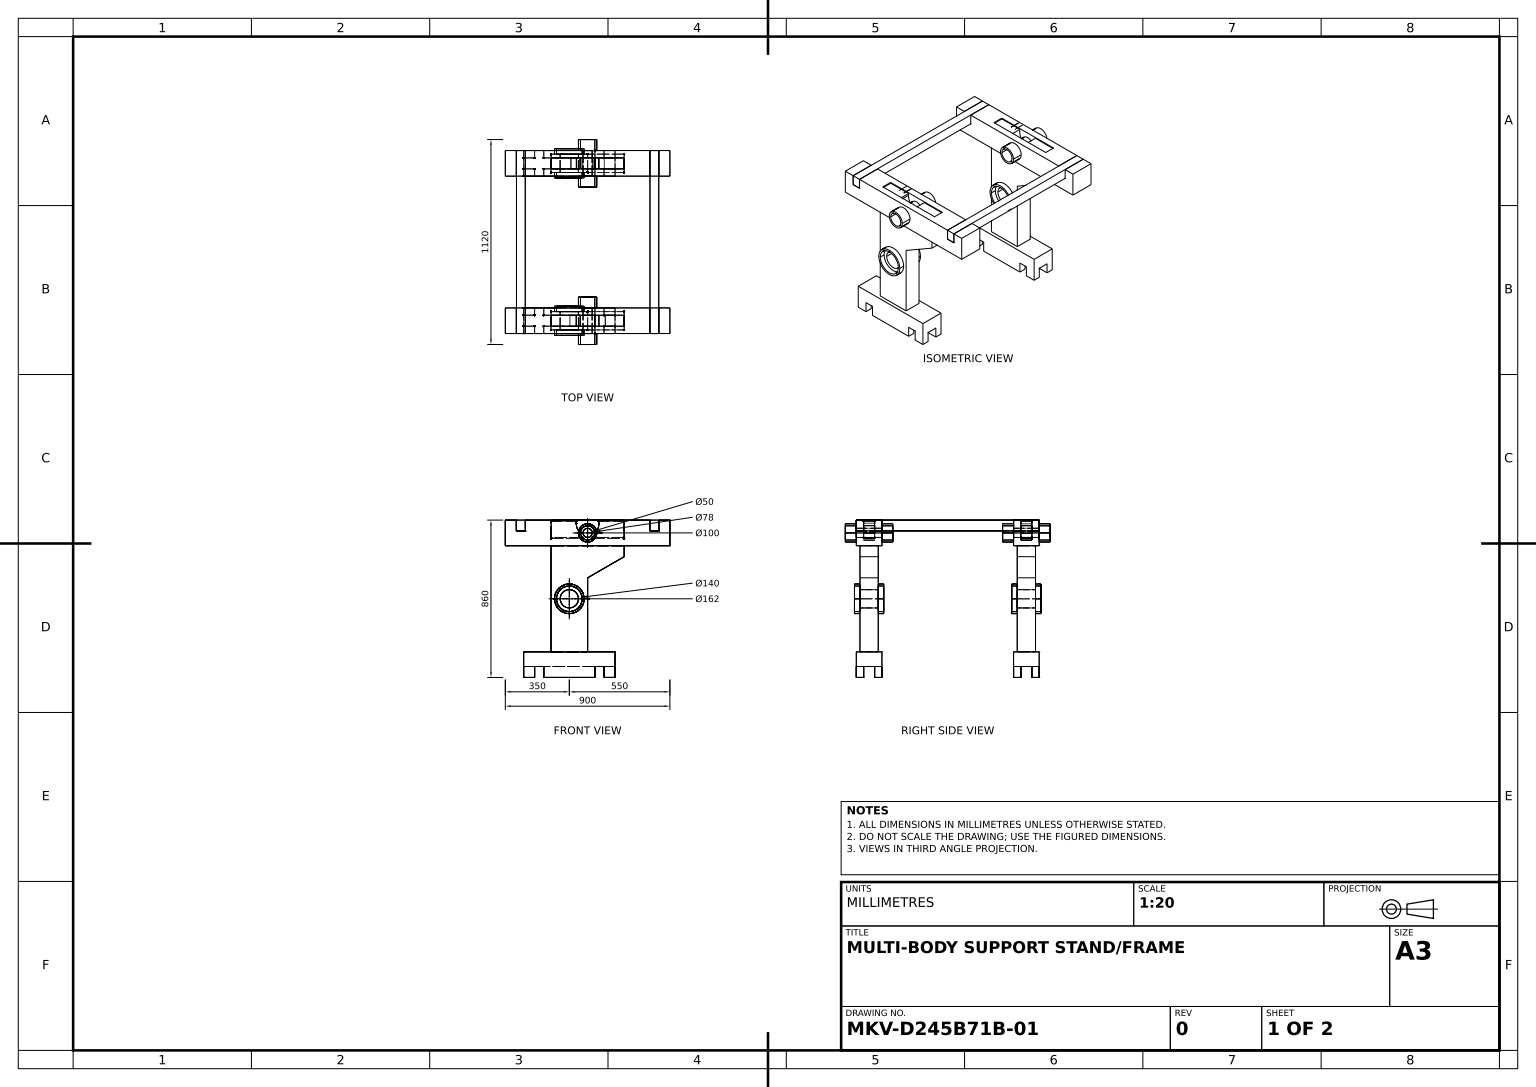
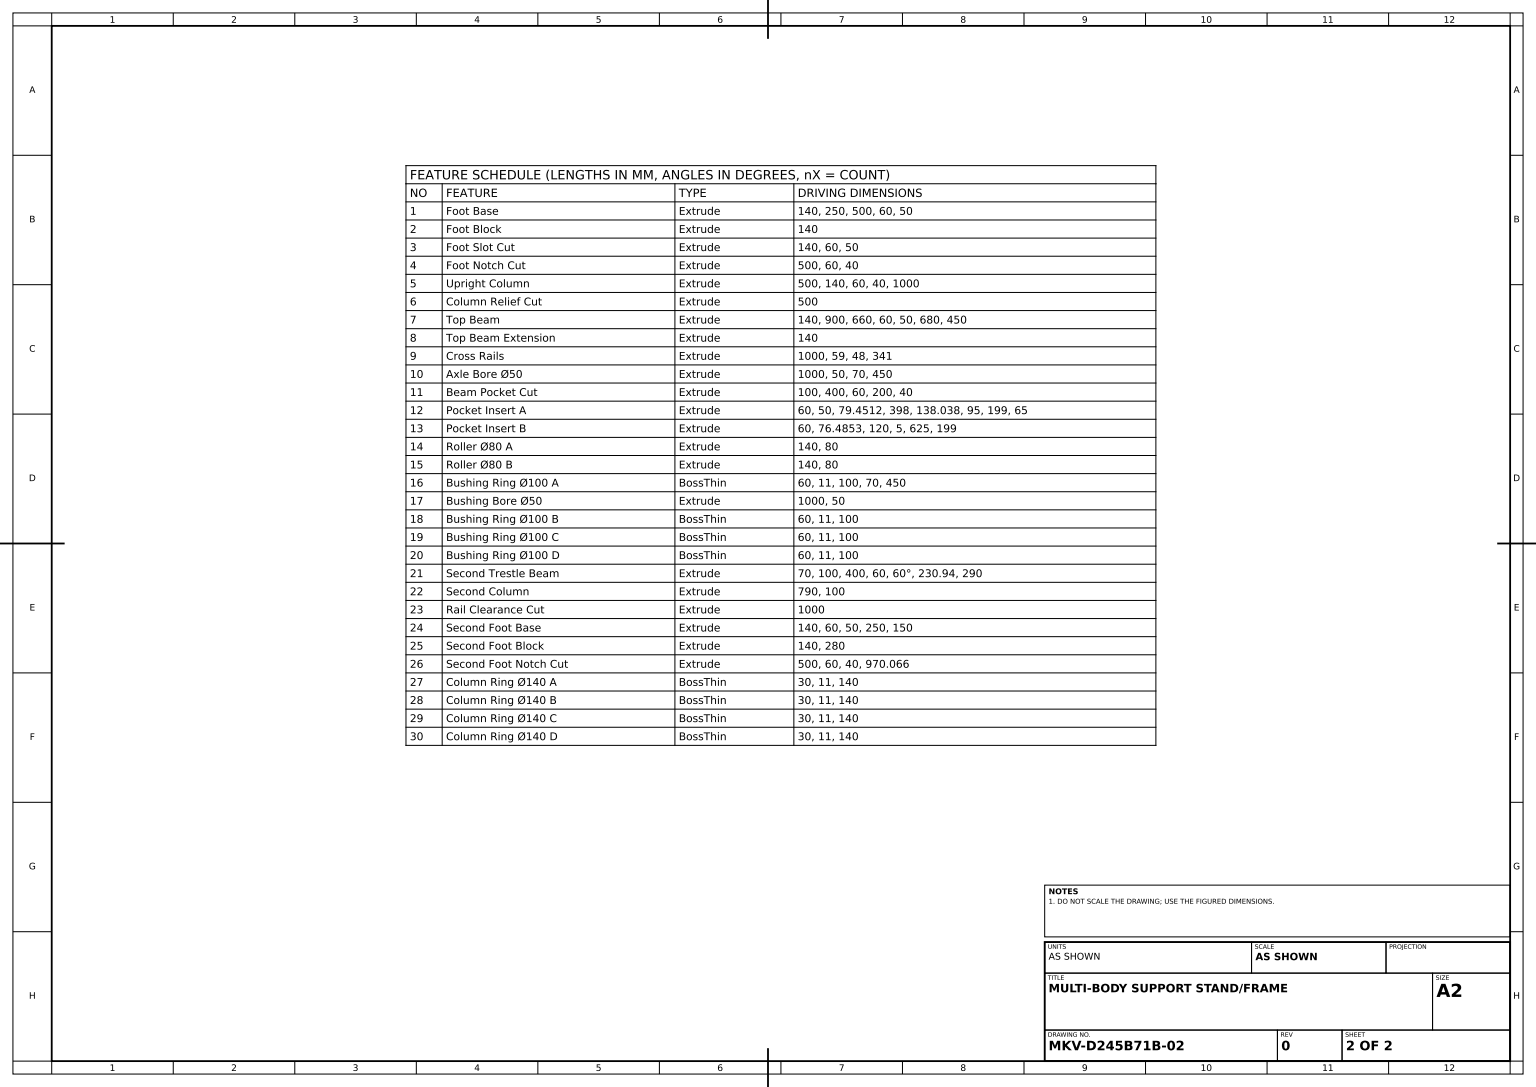
from build123d import *

# Parameters (mm, degrees)
FOOT_BASE_DEPTH               = 140
FOOT_BLOCK_SKETCH_W           = 500
FOOT_BLOCK_SKETCH_H           = 140
FOOT_BLOCK_DEPTH              = 140
FOOT_SLOT_SKETCH_W            = 50
FOOT_SLOT_SKETCH_H            = 60
FOOT_SLOT_CUT_DEPTH           = 140
FOOT_NOTCH_SKETCH_W           = 60
FOOT_NOTCH_SKETCH_H           = 60
FOOT_NOTCH_CUT_DEPTH          = 500
UPRIGHT_COLUMN_DEPTH          = 500
COLUMN_RELIEF_SKETCH_W        = 50
COLUMN_RELIEF_SKETCH_H        = 60
COLUMN_RELIEF_CUT_DEPTH       = 500
TOP_BEAM_DEPTH                = 140
TOP_BEAM_EXTENSION_DEPTH      = 140
CROSS_RAILS_SKETCH_W          = 48
CROSS_RAILS_SKETCH_H          = 59
CROSS_RAILS_DEPTH             = 1000
CROSS_RAILS_2_DEPTH           = 1000
AXLE_BORE_50_SKETCH_R         = 25
AXLE_BORE_50_DEPTH            = 1000
BEAM_POCKET_SKETCH_W          = 400
BEAM_POCKET_SKETCH_H          = 60
BEAM_POCKET_CUT_DEPTH         = 100
POCKET_INSERT_A_DEPTH         = 60
POCKET_INSERT_B_DEPTH         = 60
POCKET_INSERT_B_2_DEPTH       = 60
ROLLER_80_A_SKETCH_R          = 40
ROLLER_80_A_DEPTH             = 140
ROLLER_80_B_SKETCH_R          = 40
ROLLER_80_B_DEPTH             = 140
BUSHING_RING_100_A_SKETCH_R   = 50
BUSHING_RING_100_A_SKETCH_R_2 = 39
BUSHING_RING_100_A_DEPTH      = 60
BUSHING_BORE_50_SKETCH_R      = 25
BUSHING_BORE_50_DEPTH         = 1000
BUSHING_RING_100_B_SKETCH_R   = 50
BUSHING_RING_100_B_SKETCH_R_2 = 39
BUSHING_RING_100_B_DEPTH      = 60
BUSHING_RING_100_C_SKETCH_R   = 50
BUSHING_RING_100_C_SKETCH_R_2 = 39
BUSHING_RING_100_C_DEPTH      = 60
BUSHING_RING_100_D_SKETCH_R   = 50
BUSHING_RING_100_D_SKETCH_R_2 = 39
BUSHING_RING_100_D_DEPTH      = 60
SECOND_TRESTLE_BEAM_SKETCH_R  = 50
SECOND_TRESTLE_BEAM_DEPTH     = 50
SECOND_COLUMN_SKETCH_R        = 50
SECOND_COLUMN_DEPTH           = 50
RAIL_CLEARANCE_SKETCH_W       = 500
RAIL_CLEARANCE_SKETCH_H       = 140
RAIL_CLEARANCE_CUT_DEPTH      = 1000
SECOND_FOOT_BASE_DEPTH        = 140
SECOND_FOOT_BLOCK_DEPTH       = 140
SECOND_FOOT_NOTCH_SKETCH_W    = 60
SECOND_FOOT_NOTCH_SKETCH_H    = 60
SECOND_FOOT_NOTCH_CUT_DEPTH   = 500
COLUMN_RING_140_A_SKETCH_R    = 81
COLUMN_RING_140_A_SKETCH_R_2  = 70
COLUMN_RING_140_A_DEPTH       = 30
COLUMN_RING_140_B_SKETCH_R    = 81
COLUMN_RING_140_B_SKETCH_R_2  = 70
COLUMN_RING_140_B_DEPTH       = 30
COLUMN_RING_140_C_SKETCH_R    = 81
COLUMN_RING_140_C_SKETCH_R_2  = 70
COLUMN_RING_140_C_DEPTH       = 30
COLUMN_START                  = 30
COLUMN_RING_140_D_SKETCH_R    = 81
COLUMN_RING_140_D_SKETCH_R_2  = 70
COLUMN_RING_140_D_DEPTH       = 30


with BuildPart() as part:
    # Foot Base Sketch → Foot Base (new body)
    with BuildSketch(Plane(origin=(0, 0, 0), x_dir=(1, 0, 0), z_dir=(0, 1, 0))):
        Polygon((-250, 0), (-250, 140), (-190, 140), (-190, 80), (-140, 80), (-140, 140), (140, 140), (140, 80), (190, 80), (190, 140), (250, 140), (250, 0), align=None)
    extrude(amount=FOOT_BASE_DEPTH)

    # Foot Block Sketch → Foot Block (add)
    with BuildSketch(Plane.XY):
        with Locations((0, 70)):
            Rectangle(FOOT_BLOCK_SKETCH_W, FOOT_BLOCK_SKETCH_H)
    extrude(amount=-FOOT_BLOCK_DEPTH)

    # Foot Slot Sketch → Foot Slot Cut (cut)
    with BuildSketch(Plane.XY):
        with Locations((-165, 30)):
            Rectangle(FOOT_SLOT_SKETCH_W, FOOT_SLOT_SKETCH_H)
        with Locations((165, 30)):
            Rectangle(FOOT_SLOT_SKETCH_W, FOOT_SLOT_SKETCH_H)
    extrude(amount=-FOOT_SLOT_CUT_DEPTH, mode=Mode.SUBTRACT)

    # Foot Notch Sketch → Foot Notch Cut (cut)
    with BuildSketch(Plane.ZY.offset(250)):
        with Locations((-70, 30)):
            Rectangle(FOOT_NOTCH_SKETCH_W, FOOT_NOTCH_SKETCH_H)
    extrude(amount=-FOOT_NOTCH_CUT_DEPTH, mode=Mode.SUBTRACT)



with BuildPart() as body_2:
    # Upright Column Sketch → Upright Column (new body)
    with BuildSketch(Plane.ZY.offset(250)):
        Polygon((760, 60), (820, 60), (820, 0), (860, 0), (860, 140), (720, 140), (720, 0), (760, 0), align=None)
    extrude(amount=-UPRIGHT_COLUMN_DEPTH)

    # Column Relief Sketch → Column Relief Cut (cut)
    with BuildSketch(Plane(origin=(0, 0, 720), x_dir=(-1, 0, 0), z_dir=(0, 0, -1))):
        with Locations((-165, 30)):
            Rectangle(COLUMN_RELIEF_SKETCH_W, COLUMN_RELIEF_SKETCH_H)
        with Locations((165, 30)):
            Rectangle(COLUMN_RELIEF_SKETCH_W, COLUMN_RELIEF_SKETCH_H)
    extrude(amount=-COLUMN_RELIEF_CUT_DEPTH, mode=Mode.SUBTRACT)



with BuildPart() as body_3:
    # Top Beam Sketch → Top Beam (new body)
    with BuildSketch(Plane.XY.offset(860)):
        Polygon((450, 720), (-450, 720), (-450, 860), (-390, 860), (-390, 800), (-340, 800), (-340, 860), (340, 860), (340, 800), (390, 800), (390, 860), (450, 860), align=None)
    extrude(amount=-TOP_BEAM_DEPTH)


with BuildPart() as body_4:
    # Top Beam Extension Sketch → Top Beam Extension (new body)
    with BuildSketch(Plane(origin=(0, 0, -140), x_dir=(-1, 0, 0), z_dir=(0, 0, -1))):
        Polygon((-450, 860), (-450, 720), (450, 720), (450, 860), (390, 860), (390, 800), (340, 800), (340, 860), (-340, 860), (-340, 800), (-390, 800), (-390, 860), align=None)
    extrude(amount=-TOP_BEAM_EXTENSION_DEPTH)


with BuildPart() as body_5:
    # Cross Rails Sketch → Cross Rails (new body)
    with BuildSketch(Plane.XY.offset(860)):
        with Locations((-365, 830.5)):
            Rectangle(CROSS_RAILS_SKETCH_W, CROSS_RAILS_SKETCH_H)
    extrude(amount=-CROSS_RAILS_DEPTH)


with BuildPart() as body_6:
    # Cross Rails Sketch → Cross Rails 2 (new body)
    with BuildSketch(Plane.XY.offset(860)):
        with Locations((365, 830.5)):
            Rectangle(CROSS_RAILS_SKETCH_W, CROSS_RAILS_SKETCH_H)
    extrude(amount=-CROSS_RAILS_2_DEPTH)


with BuildPart() as axle_bore_50_tool:
    # Axle Bore Ø50 Sketch → Axle Bore Ø50 (new body)
    with BuildSketch(Plane.XY.offset(860)):
        with Locations((0, 790)):
            Circle(AXLE_BORE_50_SKETCH_R)
    extrude(amount=-AXLE_BORE_50_DEPTH)


with BuildPart() as body_3_1:
    add(body_3.part)

    # Axle Bore Ø50: cut by axle_bore_50_tool
    add(axle_bore_50_tool.part, mode=Mode.SUBTRACT)


with BuildPart() as body_4_1:
    add(body_4.part)

    # Axle Bore Ø50: cut by axle_bore_50_tool
    add(axle_bore_50_tool.part, mode=Mode.SUBTRACT)


with BuildPart() as beam_pocket_cut_tool:
    # Beam Pocket Sketch → Beam Pocket Cut (new body)
    with BuildSketch(Plane(origin=(0, 860, 0), x_dir=(1, 0, 0), z_dir=(0, 1, 0))):
        with Locations((0, -790)):
            Rectangle(BEAM_POCKET_SKETCH_W, BEAM_POCKET_SKETCH_H)
        with Locations((0, 70)):
            Rectangle(BEAM_POCKET_SKETCH_W, BEAM_POCKET_SKETCH_H)
    extrude(amount=-BEAM_POCKET_CUT_DEPTH)


with BuildPart() as body_3_2:
    add(body_3_1.part)

    # Beam Pocket Cut: cut by beam_pocket_cut_tool
    add(beam_pocket_cut_tool.part, mode=Mode.SUBTRACT)

    # Pocket Insert A Sketch → Pocket Insert A (add)
    with BuildSketch(Plane.XY.offset(760)):
        with BuildLine():
            Line((-60.961774132, 855), (-199, 855))
            Line((-199, 855), (-199, 760))
            Line((-199, 760), (199, 760))
            Line((199, 760), (199, 855))
            Line((199, 855), (60.961774132, 855))
            ThreePointArc((60.961774132, 855), (52.388331141, 804.709509525), (15, 770))
            ThreePointArc((15, 770), (7.90569415, 766.282917549), (0, 765))
            ThreePointArc((0, 765), (-7.90569415, 766.282917549), (-15, 770))
            ThreePointArc((-15, 770), (-52.388331141, 804.709509525), (-60.961774132, 855))
        make_face()
    extrude(amount=POCKET_INSERT_A_DEPTH)

    # Roller Ø80 A Sketch → Roller Ø80 A (add)
    with BuildSketch(Plane.XY.offset(860)):
        with Locations((0, 790)):
            Circle(ROLLER_80_A_SKETCH_R)
    extrude(amount=-ROLLER_80_A_DEPTH)

    # Bushing Ring Ø100 A Sketch → Bushing Ring Ø100 A (add)
    with BuildSketch(Plane.XY.offset(860)):
        with Locations((0, 790)):
            Circle(BUSHING_RING_100_A_SKETCH_R)
        with Locations((0, 790)):
            Circle(BUSHING_RING_100_A_SKETCH_R_2, mode=Mode.SUBTRACT)
    extrude(amount=BUSHING_RING_100_A_DEPTH)


with BuildPart() as body_4_2:
    add(body_4_1.part)

    # Beam Pocket Cut: cut by beam_pocket_cut_tool
    add(beam_pocket_cut_tool.part, mode=Mode.SUBTRACT)



with BuildPart() as body_7:
    # Pocket Insert B Sketch → Pocket Insert B (new body)
    with BuildSketch(Plane(origin=(0, 0, -40), x_dir=(-1, 0, 0), z_dir=(0, 0, -1))):
        with BuildLine():
            Line((-60, 855), (-199, 855))
            Line((-199, 855), (-199, 765))
            Line((-199, 765), (0, 765))
            ThreePointArc((0, 765), (-7.183697139, 766.054342869), (-13.76146789, 769.128440367))
            ThreePointArc((-13.76146789, 769.128440367), (-52.343089795, 803.738336264), (-60, 855))
        make_face()
    extrude(amount=POCKET_INSERT_B_DEPTH)


with BuildPart() as body_8:
    # Pocket Insert B Sketch → Pocket Insert B 2 (new body)
    with BuildSketch(Plane(origin=(0, 0, -40), x_dir=(-1, 0, 0), z_dir=(0, 0, -1))):
        with BuildLine():
            ThreePointArc((13.76146789, 769.128440367), (7.183697139, 766.054342869), (0, 765))
            Line((0, 765), (199, 765))
            Line((199, 765), (199, 855))
            Line((199, 855), (60, 855))
            ThreePointArc((60, 855), (52.343089795, 803.738336264), (13.76146789, 769.128440367))
        make_face()
    extrude(amount=POCKET_INSERT_B_2_DEPTH)


with BuildPart() as body_4_3:
    add(body_4_2.part)

    add(body_7.part)  # Roller Ø80 B merges body 7

    add(body_8.part)  # Roller Ø80 B merges body 8
    # Roller Ø80 B Sketch → Roller Ø80 B (add)
    with BuildSketch(Plane(origin=(0, 0, -140), x_dir=(-1, 0, 0), z_dir=(0, 0, -1))):
        with Locations((0, 790)):
            Circle(ROLLER_80_B_SKETCH_R)
    extrude(amount=-ROLLER_80_B_DEPTH)


with BuildPart() as bushing_bore_50_tool:
    # Bushing Bore Ø50 Sketch → Bushing Bore Ø50 (new body)
    with BuildSketch(Plane.XY.offset(860)):
        with Locations((0, 790)):
            Circle(BUSHING_BORE_50_SKETCH_R)
    extrude(amount=-BUSHING_BORE_50_DEPTH)


with BuildPart() as body_3_3:
    add(body_3_2.part)

    # Bushing Bore Ø50: cut by bushing_bore_50_tool
    add(bushing_bore_50_tool.part, mode=Mode.SUBTRACT)

    # Bushing Ring Ø100 B Sketch → Bushing Ring Ø100 B (add)
    with BuildSketch(Plane(origin=(0, 0, 720), x_dir=(-1, 0, 0), z_dir=(0, 0, -1))):
        with Locations((0, 790)):
            Circle(BUSHING_RING_100_B_SKETCH_R)
        with Locations((0, 790)):
            Circle(BUSHING_RING_100_B_SKETCH_R_2, mode=Mode.SUBTRACT)
    extrude(amount=BUSHING_RING_100_B_DEPTH)


with BuildPart() as body_4_4:
    add(body_4_3.part)

    # Bushing Bore Ø50: cut by bushing_bore_50_tool
    add(bushing_bore_50_tool.part, mode=Mode.SUBTRACT)

    # Bushing Ring Ø100 C Sketch → Bushing Ring Ø100 C (add)
    with BuildSketch(Plane.XY):
        with Locations((0, 790)):
            Circle(BUSHING_RING_100_C_SKETCH_R)
        with Locations((0, 790)):
            Circle(BUSHING_RING_100_C_SKETCH_R_2, mode=Mode.SUBTRACT)
    extrude(amount=BUSHING_RING_100_C_DEPTH)

    # Bushing Ring Ø100 D Sketch → Bushing Ring Ø100 D (add)
    with BuildSketch(Plane(origin=(0, 0, -140), x_dir=(-1, 0, 0), z_dir=(0, 0, -1))):
        with Locations((0, 790)):
            Circle(BUSHING_RING_100_D_SKETCH_R)
        with Locations((0, 790)):
            Circle(BUSHING_RING_100_D_SKETCH_R_2, mode=Mode.SUBTRACT)
    extrude(amount=BUSHING_RING_100_D_DEPTH)


with BuildPart() as part_1:
    add(part.part)

    add(body_4_4.part)  # Second Trestle Beam merges body 4
    # Second Trestle Beam Sketch → Second Trestle Beam (add, symmetric)
    with BuildSketch(Plane.XY.offset(-70)):
        Polygon((-200, 140), (0, 140), (0, 544.529946162), (200, 660), (200, 720), (-200, 720), align=None)
        with Locations((-100, 430)):
            Circle(SECOND_TRESTLE_BEAM_SKETCH_R, mode=Mode.SUBTRACT)
    extrude(amount=SECOND_TRESTLE_BEAM_DEPTH, both=True)


with BuildPart() as body_2_1:
    add(body_2.part)

    add(body_3_3.part)  # Second Column merges body 3
    # Second Column Sketch → Second Column (add, symmetric)
    with BuildSketch(Plane.XY.offset(790)):
        Polygon((-200, 720), (200, 720), (200, 660), (0, 544.529946162), (0, 140), (-200, 140), align=None)
        with Locations((-100, 430)):
            Circle(SECOND_COLUMN_SKETCH_R, mode=Mode.SUBTRACT)
    extrude(amount=SECOND_COLUMN_DEPTH, both=True)


with BuildPart() as rail_clearance_cut_tool:
    # Rail Clearance Sketch → Rail Clearance Cut (new body)
    with BuildSketch(Plane.XY.offset(860)):
        with Locations((0, 70)):
            Rectangle(RAIL_CLEARANCE_SKETCH_W, RAIL_CLEARANCE_SKETCH_H)
    extrude(amount=-RAIL_CLEARANCE_CUT_DEPTH)


with BuildPart() as part_2:
    add(part_1.part)

    # Rail Clearance Cut: cut by rail_clearance_cut_tool
    add(rail_clearance_cut_tool.part, mode=Mode.SUBTRACT)

    # Second Foot Block Sketch → Second Foot Block (add)
    with BuildSketch(Plane(origin=(0, 0, -140), x_dir=(-1, 0, 0), z_dir=(0, 0, -1))):
        Polygon((-150, 140), (350, 140), (350, 0), (290, 0), (290, 60), (240, 60), (240, 0), (-40, 0), (-40, 60), (-90, 60), (-90, 0), (-150, 0), align=None)
    extrude(amount=-SECOND_FOOT_BLOCK_DEPTH)


with BuildPart() as body_2_2:
    add(body_2_1.part)

    # Rail Clearance Cut: cut by rail_clearance_cut_tool
    add(rail_clearance_cut_tool.part, mode=Mode.SUBTRACT)

    # Second Foot Base Sketch → Second Foot Base (add)
    with BuildSketch(Plane.XY.offset(860)):
        Polygon((-350, 140), (-350, 0), (-290, 0), (-290, 60), (-240, 60), (-240, 0), (40, 0), (40, 60), (90, 60), (90, 0), (150, 0), (150, 140), align=None)
    extrude(amount=-SECOND_FOOT_BASE_DEPTH)


with BuildPart() as second_foot_notch_cut_tool:
    # Second Foot Notch Sketch → Second Foot Notch Cut (new body)
    with BuildSketch(Plane.ZY.offset(350)):
        with Locations((-70, 30)):
            Rectangle(SECOND_FOOT_NOTCH_SKETCH_W, SECOND_FOOT_NOTCH_SKETCH_H)
        with Locations((790, 30)):
            Rectangle(SECOND_FOOT_NOTCH_SKETCH_W, SECOND_FOOT_NOTCH_SKETCH_H)
    extrude(amount=-SECOND_FOOT_NOTCH_CUT_DEPTH)


with BuildPart() as part_3:
    add(part_2.part)

    # Second Foot Notch Cut: cut by second_foot_notch_cut_tool
    add(second_foot_notch_cut_tool.part, mode=Mode.SUBTRACT)

    # Column Ring Ø140 C Sketch → Column Ring Ø140 C (add)
    with BuildSketch(Plane.XY.offset(-20)):
        with Locations((-100, 430)):
            Circle(COLUMN_RING_140_C_SKETCH_R)
        with Locations((-100, 430)):
            Circle(COLUMN_RING_140_C_SKETCH_R_2, mode=Mode.SUBTRACT)
    extrude(amount=COLUMN_RING_140_C_DEPTH)

    # Column Ring Ø140 D Sketch → Column Ring Ø140 D (add)
    with BuildSketch(Plane(origin=(0, 0, -120), x_dir=(-1, 0, 0), z_dir=(0, 0, -1)).offset(COLUMN_START)):
        with Locations((100, 430)):
            Circle(COLUMN_RING_140_D_SKETCH_R)
        with Locations((100, 430)):
            Circle(COLUMN_RING_140_D_SKETCH_R_2, mode=Mode.SUBTRACT)
    extrude(amount=-COLUMN_RING_140_D_DEPTH)


with BuildPart() as body_2_3:
    add(body_2_2.part)

    # Second Foot Notch Cut: cut by second_foot_notch_cut_tool
    add(second_foot_notch_cut_tool.part, mode=Mode.SUBTRACT)

    # Column Ring Ø140 A Sketch → Column Ring Ø140 A (add)
    with BuildSketch(Plane.XY.offset(840)):
        with Locations((-100, 430)):
            Circle(COLUMN_RING_140_A_SKETCH_R)
        with Locations((-100, 430)):
            Circle(COLUMN_RING_140_A_SKETCH_R_2, mode=Mode.SUBTRACT)
    extrude(amount=COLUMN_RING_140_A_DEPTH)

    # Column Ring Ø140 B Sketch → Column Ring Ø140 B (add)
    with BuildSketch(Plane(origin=(0, 0, 740), x_dir=(-1, 0, 0), z_dir=(0, 0, -1))):
        with Locations((100, 430)):
            Circle(COLUMN_RING_140_B_SKETCH_R)
        with Locations((100, 430)):
            Circle(COLUMN_RING_140_B_SKETCH_R_2, mode=Mode.SUBTRACT)
    extrude(amount=COLUMN_RING_140_B_DEPTH)


solid = Compound([body_5.part, body_6.part, part_3.part, body_2_3.part])
